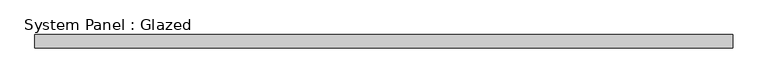
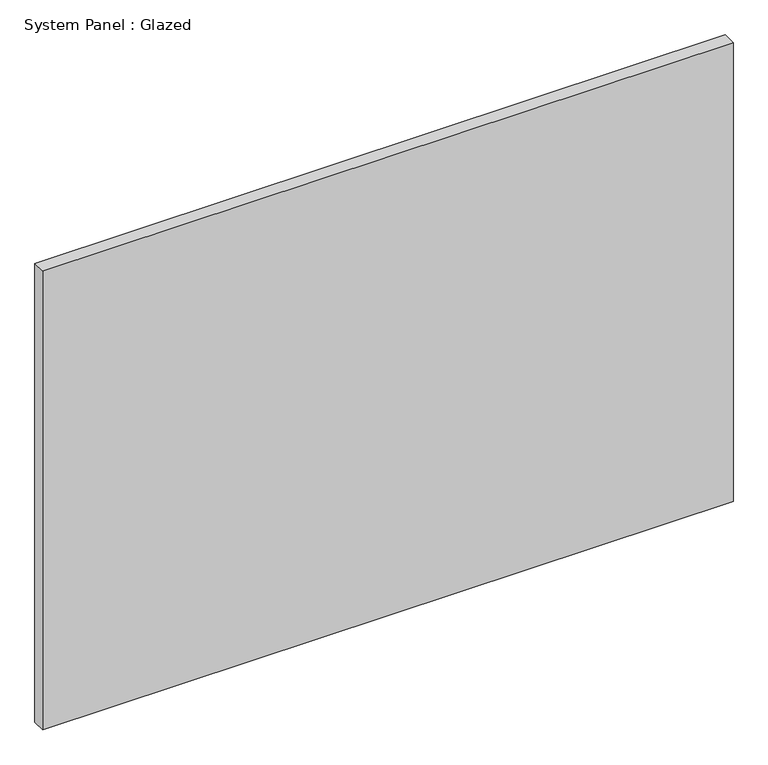
"""IFC4 building model written with IfcOpenShell, lengths in millimetres: plate geometry, System Panel : Glazed."""

from ifc_helpers import new_model, si_unit, origin, origin_with_axes, place, context, project, spatial, polyline, outline, extrude, source, transform, mapped, element, save


def system_panel_glazed_751bbe7c(model_context):
    return source(origin(), model_context, "Body", "SweptSolid", [
        extrude(outline(polyline([(655.1083334, 19.05), (-655.1083334, 19.05), (-655.1083334, 44.45), (655.1083334, 44.45), (655.1083334, 19.05)])), origin_with_axes(), (0.0, 0.0, 1.0), 920.75),
    ])


if __name__ == "__main__":
    model = new_model("IFC4")
    model_context = context("Model", 3, world=origin())
    ifc_project = project(units=[si_unit("LENGTHUNIT", "METRE", prefix="MILLI")], contexts=[model_context])
    site = spatial("IfcSite", under=ifc_project)
    building = spatial("IfcBuilding", under=site)
    placement = place(None, origin())
    system_panel_glazed_shape = system_panel_glazed_751bbe7c(model_context)
    element("IfcPlate", 1, ObjectType="System Panel : Glazed", at=placement, inside=building, context=model_context, shape_type="MappedRepresentation", body=[
        mapped(system_panel_glazed_shape, transform((0.0, 0.0, 0.0), x_axis=(1.0, 0.0, 0.0), y_axis=(0.0, 1.0, 0.0), z_axis=(0.0, 0.0, 1.0))),
    ])
    save(model, "model.ifc")

# Revit data of these elements
# Type "System Panel : Glazed"
#   Construction Type Id = "GSP4R"
#   Analytic Construction = "1/8 in Pilkington single glazing"
#   Visual Light Transmittance = 0.9
#   Solar Heat Gain Coefficient = 0.86
#   Heat Transfer Coefficient (U) = 1.18115 BTU/(h·ft²·°F)
#   Define Thermal Properties by = 1
# Element 1 (IfcPlate, "System Panel : Glazed")
#   Materials on its faces: "glass panel 223"
# Materials
#   "glass panel 223": class "Generic", colour RGB 120 120 120, transparency 0, Cost = 0
